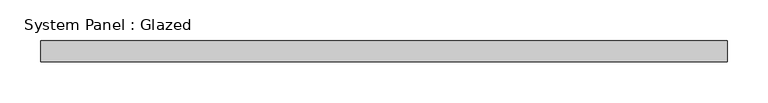
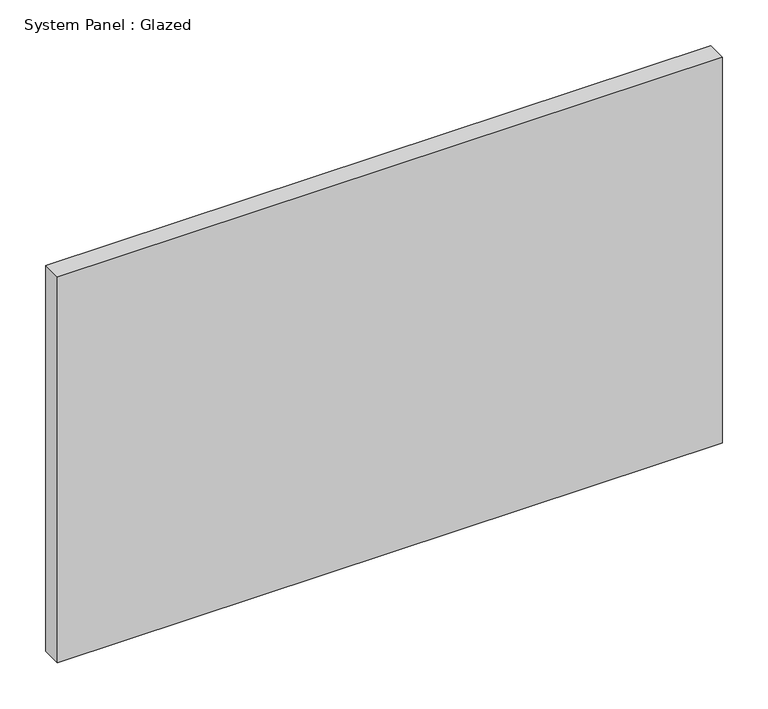
"""IFC4 building model written with IfcOpenShell, lengths in millimetres: plate geometry, System Panel : Glazed."""

from ifc_helpers import new_model, si_unit, origin, origin_with_axes, place, context, project, spatial, polyline, outline, extrude, source, transform, mapped, element, save


def system_panel_glazed_73486e20(model_context):
    return source(origin(), model_context, "Body", "SweptSolid", [
        extrude(outline(polyline([(419.1, 19.05), (-419.1, 19.05), (-419.1, 44.45), (419.1, 44.45), (419.1, 19.05)])), origin_with_axes(), (0.0, 0.0, 1.0), 514.35),
    ])


if __name__ == "__main__":
    model = new_model("IFC4")
    model_context = context("Model", 3, world=origin())
    ifc_project = project(units=[si_unit("LENGTHUNIT", "METRE", prefix="MILLI")], contexts=[model_context])
    site = spatial("IfcSite", under=ifc_project)
    building = spatial("IfcBuilding", under=site)
    placement = place(None, origin())
    system_panel_glazed_shape = system_panel_glazed_73486e20(model_context)
    element("IfcPlate", 1, ObjectType="System Panel : Glazed", at=placement, inside=building, context=model_context, shape_type="MappedRepresentation", body=[
        mapped(system_panel_glazed_shape, transform((0.0, 0.0, 0.0), x_axis=(1.0, 0.0, 0.0), y_axis=(0.0, 1.0, 0.0), z_axis=(0.0, 0.0, 1.0))),
    ])
    save(model, "model.ifc")

# Revit data of these elements
# Type "System Panel : Glazed"
#   Construction Type Id = "GSP4R"
#   Analytic Construction = "1/8 in Pilkington single glazing"
#   Visual Light Transmittance = 0.9
#   Solar Heat Gain Coefficient = 0.86
#   Heat Transfer Coefficient (U) = 1.18115 BTU/(h·ft²·°F)
#   Define Thermal Properties by = 1
# Element 1 (IfcPlate, "System Panel : Glazed")
#   Materials on its faces: "glass panel 223"
# Materials
#   "glass panel 223": class "Generic", colour RGB 120 120 120, transparency 0, Cost = 0
